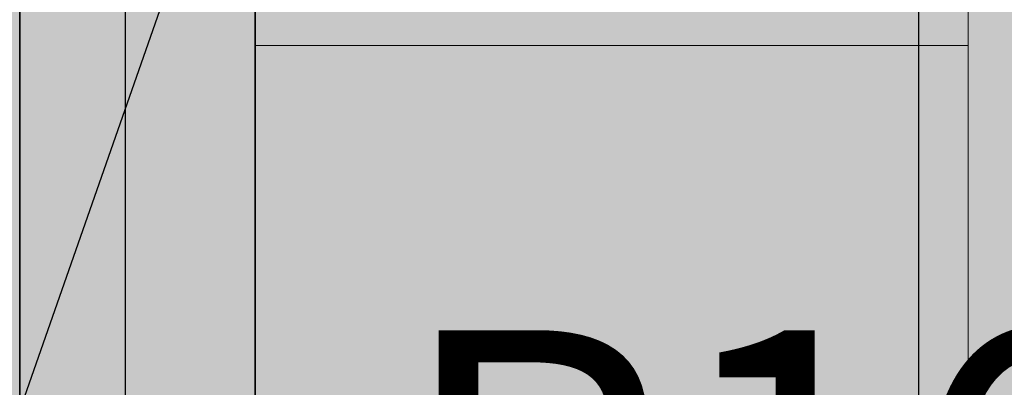
# Model space of a CAD drawing. Units: millimetres. Extents: x 130 to 1021, y 147 to 699.
# Tile 33 of 40: x 487 to 550, y 515 to 539. Entities that reach past the tile are written whole.
import ezdxf

# ---------------------------------------------------------------- set-up
doc = ezdxf.new("R2010")
doc.units = ezdxf.units.MM
doc.header["$MEASUREMENT"] = 0
for name, color, linetype, lineweight in [('A-ANNO-DIMS', 2, 'Continuous', 18), ('A-ELEV', 7, 'Continuous', 35), ('A-ELEV-PATT', 9, 'Continuous', 13), ('A-GLAZ', 4, 'Continuous', 18)]:
    doc.layers.add(name, color=color, linetype=linetype, lineweight=lineweight)
doc.styles.get("Standard").update_dxf_attribs({"font": 'arial.ttf'})
doc.dimstyles.get("Standard").update_dxf_attribs({"dimtxt": 20, "dimasz": 10, "dimexe": 10, "dimexo": 10, "dimgap": 5, "dimtad": 0, "dimtih": 1, "dimtoh": 1, "dimdec": 0, "dimzin": 0, "dimdsep": 46, "dimtxsty": 'Standard', "dimcen": 5, "dimadec": 0, "dimazin": 0, "dimtfac": 1, "dimtdec": 0, "dimtofl": 0, "dimtmove": 0, "dimatfit": 3, "dimfxl": 1, "dimtolj": 1, "dimtzin": 0, "dimarcsym": 0})

# ---------------------------------------------------------------- blocks, each defined once
blk = doc.blocks.new('*D11')
at = {"layer": 'A-ANNO-DIMS', "color": 0, "lineweight": -2, "transparency": 16777216}
for p, q in [((737.374, 648.699), (737.374, 149.739)), ((299.374, 566.947), (299.374, 149.739)), ((309.374, 159.739), (490.857, 159.739)), ((727.374, 159.739), (545.891, 159.739))]:
    blk.add_line(p, q, dxfattribs=at)
at = {"layer": 'A-ANNO-DIMS', "color": 0, "transparency": 16777216}
for points in [[(309.374, 161.406), (309.374, 158.073), (299.374, 159.739)], [(727.374, 161.406), (727.374, 158.073), (737.374, 159.739)]]:
    blk.add_solid(points, dxfattribs=at)
at = {"layer": 'Defpoints', "color": 0, "transparency": 16777216}
for p in [(737.374, 658.699), (299.374, 576.947), (737.374, 159.739)]:
    blk.add_point(p, dxfattribs=at)
at = {"layer": 'A-ANNO-DIMS', "color": 0, "transparency": 16777216, "insert": (518.374, 159.739), "char_height": 20, "attachment_point": 5}
blk.add_mtext('\\A1;438', dxfattribs=at)
blk = doc.blocks.new('*D12')
at = {"layer": 'A-ANNO-DIMS', "color": 0, "lineweight": -2, "transparency": 16777216}
for p, q in [((477.374, 661.947), (265.074, 661.947)), ((275.074, 651.947), (275.074, 438.205)), ((275.074, 194.039), (275.074, 407.782)), ((357.163, 184.039), (265.074, 184.039))]:
    blk.add_line(p, q, dxfattribs=at)
at = {"layer": 'A-ANNO-DIMS', "color": 0, "transparency": 16777216}
for points in [[(273.407, 651.947), (276.74, 651.947), (275.074, 661.947)], [(273.407, 194.039), (276.74, 194.039), (275.074, 184.039)]]:
    blk.add_solid(points, dxfattribs=at)
at = {"layer": 'Defpoints', "color": 0, "transparency": 16777216}
for p in [(275.074, 661.947), (487.374, 661.947), (367.163, 184.039)]:
    blk.add_point(p, dxfattribs=at)
at = {"layer": 'A-ANNO-DIMS', "color": 0, "transparency": 16777216, "insert": (275.074, 422.993), "char_height": 20, "attachment_point": 5}
blk.add_mtext('\\A1;477.9', dxfattribs=at)
blk = doc.blocks.new('*D19')
at = {"layer": 'A-ANNO-DIMS', "color": 0, "lineweight": -2, "transparency": 16777216}
for p, q in [((382.374, 388.947), (382.374, 696.247)), ((414.652, 510.881), (414.652, 696.247)), ((392.374, 686.247), (404.652, 686.247)), ((414.652, 686.247), (424.652, 686.247))]:
    blk.add_line(p, q, dxfattribs=at)
at = {"layer": 'A-ANNO-DIMS', "color": 0, "transparency": 16777216}
for points in [[(392.374, 687.914), (392.374, 684.581), (382.374, 686.247)], [(404.652, 687.914), (404.652, 684.581), (414.652, 686.247)]]:
    blk.add_solid(points, dxfattribs=at)
at = {"layer": 'Defpoints', "color": 0, "transparency": 16777216}
for p in [(414.652, 686.247), (414.652, 500.881), (382.374, 378.947)]:
    blk.add_point(p, dxfattribs=at)
at = {"layer": 'A-ANNO-DIMS', "color": 0, "transparency": 16777216, "insert": (463.411, 686.247), "char_height": 20, "attachment_point": 5}
blk.add_mtext('\\A1;32.28', dxfattribs=at)
blk = doc.blocks.new('*D20')
at = {"layer": 'A-ANNO-DIMS', "color": 0, "lineweight": -2, "transparency": 16777216}
for p, q in [((414.652, 510.881), (414.652, 696.247)), ((432.374, 388.947), (432.374, 696.247)), ((404.652, 686.247), (394.652, 686.247)), ((442.374, 686.247), (452.374, 686.247))]:
    blk.add_line(p, q, dxfattribs=at)
at = {"layer": 'A-ANNO-DIMS', "color": 0, "transparency": 16777216}
for points in [[(404.652, 687.914), (404.652, 684.581), (414.652, 686.247)], [(442.374, 687.914), (442.374, 684.581), (432.374, 686.247)]]:
    blk.add_solid(points, dxfattribs=at)
at = {"layer": 'Defpoints', "color": 0, "transparency": 16777216}
for p in [(432.374, 686.247), (414.652, 500.881), (432.374, 378.947)]:
    blk.add_point(p, dxfattribs=at)
at = {"layer": 'A-ANNO-DIMS', "color": 0, "transparency": 16777216, "insert": (490.075, 686.247), "char_height": 20, "attachment_point": 5}
blk.add_mtext('\\A1;17.72', dxfattribs=at)
blk = doc.blocks.new('*D21')
at = {"layer": 'A-ANNO-DIMS', "color": 0, "lineweight": -2, "transparency": 16777216}
for p, q in [((432.374, 388.947), (432.374, 696.247)), ((447.374, 656.947), (447.374, 696.247)), ((422.374, 686.247), (412.374, 686.247)), ((457.374, 686.247), (467.374, 686.247))]:
    blk.add_line(p, q, dxfattribs=at)
at = {"layer": 'A-ANNO-DIMS', "color": 0, "transparency": 16777216}
for points in [[(422.374, 687.914), (422.374, 684.581), (432.374, 686.247)], [(457.374, 687.914), (457.374, 684.581), (447.374, 686.247)]]:
    blk.add_solid(points, dxfattribs=at)
at = {"layer": 'Defpoints', "color": 0, "transparency": 16777216}
for p in [(447.374, 686.247), (447.374, 646.947), (432.374, 378.947)]:
    blk.add_point(p, dxfattribs=at)
at = {"layer": 'A-ANNO-DIMS', "color": 0, "transparency": 16777216, "insert": (485.832, 686.247), "char_height": 20, "attachment_point": 5}
blk.add_mtext('\\A1;15', dxfattribs=at)
blk = doc.blocks.new('*D22')
at = {"layer": 'A-ANNO-DIMS', "color": 0, "lineweight": -2, "transparency": 16777216}
for p, q in [((447.374, 656.947), (447.374, 696.247)), ((466.767, 403.947), (466.767, 696.247)), ((437.374, 686.247), (427.374, 686.247)), ((476.767, 686.247), (486.767, 686.247))]:
    blk.add_line(p, q, dxfattribs=at)
at = {"layer": 'A-ANNO-DIMS', "color": 0, "transparency": 16777216}
for points in [[(437.374, 687.914), (437.374, 684.581), (447.374, 686.247)], [(476.767, 687.914), (476.767, 684.581), (466.767, 686.247)]]:
    blk.add_solid(points, dxfattribs=at)
at = {"layer": 'Defpoints', "color": 0, "transparency": 16777216}
for p in [(466.767, 686.247), (447.374, 646.947), (466.767, 393.947)]:
    blk.add_point(p, dxfattribs=at)
at = {"layer": 'A-ANNO-DIMS', "color": 0, "transparency": 16777216, "insert": (532.34, 686.247), "char_height": 20, "attachment_point": 5}
blk.add_mtext('\\A1;19.393', dxfattribs=at)
blk = doc.blocks.new('*D23')
at = {"layer": 'A-ANNO-DIMS', "color": 0, "lineweight": -2, "transparency": 16777216}
for p, q in [((466.767, 403.947), (466.767, 696.247)), ((475.988, 209.039), (475.988, 696.247)), ((456.767, 686.247), (446.767, 686.247)), ((485.988, 686.247), (495.988, 686.247))]:
    blk.add_line(p, q, dxfattribs=at)
at = {"layer": 'A-ANNO-DIMS', "color": 0, "transparency": 16777216}
for points in [[(456.767, 687.914), (456.767, 684.581), (466.767, 686.247)], [(485.988, 687.914), (485.988, 684.581), (475.988, 686.247)]]:
    blk.add_solid(points, dxfattribs=at)
at = {"layer": 'Defpoints', "color": 0, "transparency": 16777216}
for p in [(475.988, 686.247), (466.767, 393.947), (475.988, 199.039)]:
    blk.add_point(p, dxfattribs=at)
at = {"layer": 'A-ANNO-DIMS', "color": 0, "transparency": 16777216, "insert": (534.631, 686.247), "char_height": 20, "attachment_point": 5}
blk.add_mtext('\\A1;9.222', dxfattribs=at)
blk = doc.blocks.new('*D24')
at = {"layer": 'A-ANNO-DIMS', "color": 0, "lineweight": -2, "transparency": 16777216}
for p, q in [((475.988, 209.039), (475.988, 696.247)), ((487.374, 671.947), (487.374, 696.247)), ((465.988, 686.247), (455.988, 686.247)), ((497.374, 686.247), (507.374, 686.247))]:
    blk.add_line(p, q, dxfattribs=at)
at = {"layer": 'A-ANNO-DIMS', "color": 0, "transparency": 16777216}
for points in [[(465.988, 687.914), (465.988, 684.581), (475.988, 686.247)], [(497.374, 687.914), (497.374, 684.581), (487.374, 686.247)]]:
    blk.add_solid(points, dxfattribs=at)
at = {"layer": 'Defpoints', "color": 0, "transparency": 16777216}
for p in [(487.374, 686.247), (487.374, 661.947), (475.988, 199.039)]:
    blk.add_point(p, dxfattribs=at)
at = {"layer": 'A-ANNO-DIMS', "color": 0, "transparency": 16777216, "insert": (553.022, 686.247), "char_height": 20, "attachment_point": 5}
blk.add_mtext('\\A1;11.385', dxfattribs=at)
blk = doc.blocks.new('*D25')
at = {"layer": 'A-ANNO-DIMS', "color": 0, "lineweight": -2, "transparency": 16777216}
for p, q in [((487.374, 671.947), (487.374, 696.247)), ((494.102, 506.908), (494.102, 696.247)), ((477.374, 686.247), (467.374, 686.247)), ((504.102, 686.247), (514.102, 686.247))]:
    blk.add_line(p, q, dxfattribs=at)
at = {"layer": 'A-ANNO-DIMS', "color": 0, "transparency": 16777216}
for points in [[(477.374, 687.914), (477.374, 684.581), (487.374, 686.247)], [(504.102, 687.914), (504.102, 684.581), (494.102, 686.247)]]:
    blk.add_solid(points, dxfattribs=at)
at = {"layer": 'Defpoints', "color": 0, "transparency": 16777216}
for p in [(494.102, 686.247), (487.374, 661.947), (494.102, 496.908)]:
    blk.add_point(p, dxfattribs=at)
at = {"layer": 'A-ANNO-DIMS', "color": 0, "transparency": 16777216, "insert": (552.922, 686.247), "char_height": 20, "attachment_point": 5}
blk.add_mtext('\\A1;6.728', dxfattribs=at)
blk = doc.blocks.new('*D26')
at = {"layer": 'A-ANNO-DIMS', "color": 0, "lineweight": -2, "transparency": 16777216}
for p, q in [((494.102, 506.908), (494.102, 696.247)), ((502.374, 593.947), (502.374, 696.247)), ((484.102, 686.247), (474.102, 686.247)), ((512.374, 686.247), (522.374, 686.247))]:
    blk.add_line(p, q, dxfattribs=at)
at = {"layer": 'A-ANNO-DIMS', "color": 0, "transparency": 16777216}
for points in [[(484.102, 687.914), (484.102, 684.581), (494.102, 686.247)], [(512.374, 687.914), (512.374, 684.581), (502.374, 686.247)]]:
    blk.add_solid(points, dxfattribs=at)
at = {"layer": 'Defpoints', "color": 0, "transparency": 16777216}
for p in [(502.374, 686.247), (502.374, 583.947), (494.102, 496.908)]:
    blk.add_point(p, dxfattribs=at)
at = {"layer": 'A-ANNO-DIMS', "color": 0, "transparency": 16777216, "insert": (561.03, 686.247), "char_height": 20, "attachment_point": 5}
blk.add_mtext('\\A1;8.272', dxfattribs=at)
blk = doc.blocks.new('*D27')
at = {"layer": 'A-ANNO-DIMS', "color": 0, "lineweight": -2, "transparency": 16777216}
for p, q in [((502.374, 593.947), (502.374, 696.247)), ((544.635, 396.264), (544.635, 696.247)), ((512.374, 686.247), (534.635, 686.247)), ((544.635, 686.247), (554.635, 686.247))]:
    blk.add_line(p, q, dxfattribs=at)
at = {"layer": 'A-ANNO-DIMS', "color": 0, "transparency": 16777216}
for points in [[(512.374, 687.914), (512.374, 684.581), (502.374, 686.247)], [(534.635, 687.914), (534.635, 684.581), (544.635, 686.247)]]:
    blk.add_solid(points, dxfattribs=at)
at = {"layer": 'Defpoints', "color": 0, "transparency": 16777216}
for p in [(544.635, 686.247), (502.374, 583.947), (544.635, 386.264)]:
    blk.add_point(p, dxfattribs=at)
at = {"layer": 'A-ANNO-DIMS', "color": 0, "transparency": 16777216, "insert": (593.776, 686.247), "char_height": 20, "attachment_point": 5}
blk.add_mtext('\\A1;42.26', dxfattribs=at)
blk = doc.blocks.new('*D28')
at = {"layer": 'A-ANNO-DIMS', "color": 0, "lineweight": -2, "transparency": 16777216}
for p, q in [((544.635, 396.264), (544.635, 696.247)), ((552.374, 593.947), (552.374, 696.247)), ((534.635, 686.247), (524.635, 686.247)), ((562.374, 686.247), (572.374, 686.247))]:
    blk.add_line(p, q, dxfattribs=at)
at = {"layer": 'A-ANNO-DIMS', "color": 0, "transparency": 16777216}
for points in [[(534.635, 687.914), (534.635, 684.581), (544.635, 686.247)], [(562.374, 687.914), (562.374, 684.581), (552.374, 686.247)]]:
    blk.add_solid(points, dxfattribs=at)
at = {"layer": 'Defpoints', "color": 0, "transparency": 16777216}
for p in [(552.374, 686.247), (552.374, 583.947), (544.635, 386.264)]:
    blk.add_point(p, dxfattribs=at)
at = {"layer": 'A-ANNO-DIMS', "color": 0, "transparency": 16777216, "insert": (611.057, 686.247), "char_height": 20, "attachment_point": 5}
blk.add_mtext('\\A1;7.738', dxfattribs=at)
blk = doc.blocks.new('*D65')
at = {"layer": 'A-ANNO-DIMS', "color": 0, "lineweight": -2, "transparency": 16777216}
for p, q in [((495.463, 509.127), (472.508, 423.108)), ((505.463, 509.127), (495.463, 509.127)), ((427.374, 248.979), (427.374, 258.979)), ((422.374, 253.979), (432.374, 253.979))]:
    blk.add_line(p, q, dxfattribs=at)
at = {"layer": 'A-ANNO-DIMS', "color": 0, "transparency": 16777216}
blk.add_solid([(470.898, 423.538), (474.118, 422.679), (469.93, 413.447)], dxfattribs=at)
at = {"layer": 'Defpoints', "color": 0, "transparency": 16777216}
for p in [(469.93, 413.447), (427.374, 253.979)]:
    blk.add_point(p, dxfattribs=at)
at = {"layer": 'A-ANNO-DIMS', "color": 0, "transparency": 16777216, "insert": (561.623, 509.127), "char_height": 20, "attachment_point": 5}
blk.add_mtext('\\A1;R165.05', dxfattribs=at)
blk = doc.blocks.new('*D69')
at = {"layer": 'A-ANNO-DIMS', "color": 0, "lineweight": -2, "transparency": 16777216}
for p, q in [((507.746, 572.261), (483.091, 501.813)), ((517.746, 572.261), (507.746, 572.261)), ((433.191, 354.23), (433.191, 364.23)), ((428.191, 359.23), (438.191, 359.23))]:
    blk.add_line(p, q, dxfattribs=at)
at = {"layer": 'A-ANNO-DIMS', "color": 0, "transparency": 16777216}
blk.add_solid([(481.518, 502.363), (484.664, 501.262), (479.788, 492.374)], dxfattribs=at)
at = {"layer": 'Defpoints', "color": 0, "transparency": 16777216}
for p in [(479.788, 492.374), (433.191, 359.23)]:
    blk.add_point(p, dxfattribs=at)
at = {"layer": 'A-ANNO-DIMS', "color": 0, "transparency": 16777216, "insert": (573.824, 572.261), "char_height": 20, "attachment_point": 5}
blk.add_mtext('\\A1;R141.06', dxfattribs=at)
blk = doc.blocks.new('*D71')
at = {"layer": 'A-ANNO-DIMS', "color": 0, "lineweight": -2, "transparency": 16777216}
for p, q in [((492.108, 581.609), (472.542, 512.666)), ((502.108, 581.609), (492.108, 581.609)), ((432.65, 367.109), (432.65, 377.109)), ((427.65, 372.109), (437.65, 372.109))]:
    blk.add_line(p, q, dxfattribs=at)
at = {"layer": 'A-ANNO-DIMS', "color": 0, "transparency": 16777216}
blk.add_solid([(470.938, 513.121), (474.145, 512.211), (469.812, 503.046)], dxfattribs=at)
at = {"layer": 'Defpoints', "color": 0, "transparency": 16777216}
for p in [(469.812, 503.046), (432.65, 372.109)]:
    blk.add_point(p, dxfattribs=at)
at = {"layer": 'A-ANNO-DIMS', "color": 0, "transparency": 16777216, "insert": (548.493, 581.609), "char_height": 20, "attachment_point": 5}
blk.add_mtext('\\A1;R136.1', dxfattribs=at)
blk = doc.blocks.new('*D72')
at = {"layer": 'A-ANNO-DIMS', "color": 0, "lineweight": -2, "transparency": 16777216}
for p, q in [((460.658, 573.64), (451.279, 503.49)), ((470.658, 573.64), (460.658, 573.64)), ((432.115, 355.142), (432.115, 365.142)), ((427.115, 360.142), (437.115, 360.142))]:
    blk.add_line(p, q, dxfattribs=at)
at = {"layer": 'A-ANNO-DIMS', "color": 0, "transparency": 16777216}
blk.add_solid([(449.628, 503.711), (452.931, 503.27), (449.954, 493.579)], dxfattribs=at)
at = {"layer": 'Defpoints', "color": 0, "transparency": 16777216}
for p in [(449.954, 493.579), (432.115, 360.142)]:
    blk.add_point(p, dxfattribs=at)
at = {"layer": 'A-ANNO-DIMS', "color": 0, "transparency": 16777216, "insert": (526.64, 573.64), "char_height": 20, "attachment_point": 5}
blk.add_mtext('\\A1;R134.62', dxfattribs=at)

msp = doc.modelspace()

# ---------------------------------------------------------------- hatches: boundary and pattern name
at = {"layer": 'A-ELEV-PATT'}
h = msp.add_hatch(color=256, dxfattribs=at)
h.paths.add_polyline_path([(327.3738, 569.884), (327.3738, 573.9473), (307.3738, 573.9473), (307.3738, 476.9473), (327.3738, 476.9473), (327.3738, 480.95)])
h.paths.add_polyline_path([(486.7667, 386.2639), (486.7667, 393.9473), (466.7667, 393.9473), (466.7667, 357.2114), (466.7667, 311.9335, 0.0342703), (486.7667, 308.4637)])
h.paths.add_polyline_path([(486.7667, 308.4637, -0.0342703), (466.7667, 311.9335), (466.7667, 273.9473), (486.7667, 273.9473)])
h.paths.add_polyline_path([(389.3738, 351.5473), (396.7693, 351.5473, -0.007027), (393.8774, 354.5473), (389.3738, 354.5473), (389.3738, 359.5775, -0.0190302), (382.3738, 368.424), (382.3738, 249.5473), (432.3738, 249.5473), (432.3738, 325.067, -0.0057673), (429.3738, 326.709), (429.3738, 257.5473), (426.3738, 257.5473), (426.3738, 328.4428, -0.0059254), (423.3738, 330.272), (423.3738, 315.7473), (389.3738, 315.7473), (389.3738, 332.1473), (420.4552, 332.1473, -0.008951), (416.0768, 335.1473), (389.3738, 335.1473)])
h.paths.add_polyline_path([(389.3738, 312.7473), (423.3738, 312.7473), (423.3738, 296.3473), (389.3738, 296.3473)], flags=16)
h.paths.add_polyline_path([(389.3738, 293.3473), (423.3738, 293.3473), (423.3738, 276.9473), (389.3738, 276.9473)], flags=16)
h.paths.add_polyline_path([(389.3738, 273.9473), (423.3738, 273.9473), (423.3738, 257.5473), (389.3738, 257.5473)], flags=16)
h.paths.add_polyline_path([(432.3738, 378.9473), (382.3738, 378.9473), (382.3738, 368.424, 0.0190302), (389.3738, 359.5775), (389.3738, 370.9473), (423.3738, 370.9473), (423.3738, 354.5473), (393.8774, 354.5473, 0.007027), (396.7693, 351.5473), (423.3738, 351.5473), (423.3738, 335.1473), (416.0768, 335.1473, 0.008951), (420.4552, 332.1473), (423.3738, 332.1473), (423.3738, 330.272, 0.0059254), (426.3738, 328.4428), (426.3738, 370.9473), (429.3738, 370.9473), (429.3738, 326.709, 0.0057673), (432.3738, 325.067)])
h.paths.add_polyline_path([(466.7667, 357.2114), (466.7667, 393.9473), (447.3738, 393.9473), (447.3738, 357.2114), (447.3738, 318.1243, 0.0063261), (450.8779, 316.785), (450.8779, 331.5915), (463.5608, 331.5915), (463.5608, 312.7571, 0.005582), (466.7667, 311.9335)])
h.paths.add_polyline_path([(450.8779, 334.5915), (450.8779, 360.0915), (463.5608, 360.0915), (463.5608, 334.5915)], flags=16)
h.paths.add_polyline_path([(450.8779, 363.0915), (450.8779, 388.6449), (463.5608, 388.6449), (463.5608, 363.0915)], flags=16)
h.paths.add_polyline_path([(466.7667, 311.9335, -0.005582), (463.5608, 312.7571), (463.5608, 306.0915), (450.8779, 306.0915), (450.8779, 316.785, -0.0063261), (447.3738, 318.1243), (447.3738, 273.9473), (466.7667, 273.9473)])
h.paths.add_polyline_path([(450.8779, 303.0915), (463.5608, 303.0915), (463.5608, 277.5915), (450.8779, 277.5915)], flags=16)
h.paths.add_polyline_path([(552.3738, 357.2114), (552.3738, 393.9473), (486.7667, 393.9473), (486.7667, 386.2639), (544.6354, 386.2639), (544.6354, 280.6619), (486.7667, 280.6619), (486.7667, 273.9473), (552.3738, 273.9473)])
h.paths.add_polyline_path([(487.3738, 583.9473), (472.3738, 580.1973), (472.3738, 507.0765), (472.3738, 505.4251, -0.0056452), (475.3738, 504.4942), (475.3738, 506.3543), (475.3738, 511.9473), (484.3738, 511.9473), (484.3738, 503.8134), (484.3738, 501.2439, -0.0058357), (487.3738, 500.0015)])
h.paths.add_polyline_path([(484.3738, 578.0434), (484.3738, 548.9473), (475.3738, 548.9473), (475.3738, 575.7934)], flags=16)
h.paths.add_polyline_path([(484.3738, 546.9473), (484.3738, 513.9473), (475.3738, 513.9473), (475.3738, 518.7148), (475.3738, 546.9473)], flags=16)
for points in [[(502.3738, 583.9473), (487.3738, 583.9473), (487.3738, 500.0015, -0.0133113), (494.1023, 496.908), (494.1023, 476.9473), (502.3738, 476.9473)], [(502.3738, 583.9473), (502.3738, 577.3739), (547.7773, 577.3739), (547.7773, 481.7432), (502.3738, 481.7432), (502.3738, 476.9473), (552.3738, 476.9473), (552.3738, 583.9473)]]:
    msp.add_hatch(color=256, dxfattribs=at).paths.add_polyline_path(points)
h = msp.add_hatch(color=256, dxfattribs=at)
h.dxf.hatch_style = 1
h.paths.add_polyline_path([(502.3738, 566.2111), (502.3738, 548.9473), (547.7773, 548.9473), (547.7773, 566.2111)])
h.paths.add_polyline_path([(502.3738, 546.9473), (502.3738, 537.2685), (547.7773, 537.2685), (547.7773, 546.9473)])
h.paths.add_polyline_path([(486.7667, 360.9454), (486.7667, 336.9454), (544.6354, 336.9453), (544.6354, 360.9453)])
h.paths.add_polyline_path([(496.0546, 377.43), (486.7667, 370.4028), (486.7667, 363.9454), (544.6354, 363.9453), (544.6354, 377.43)])
h = msp.add_hatch(color=256, dxfattribs=at)
h.dxf.hatch_style = 1
h.paths.add_polyline_path([(364.0891, 218.0087), (361.0152, 221.978), (361.0152, 236.978), (357.9413, 240.9473), (357.9413, 195.9473), (367.163, 184.0395), (367.163, 199.0395), (364.0891, 203.0087)])
h.paths.add_polyline_path([(502.3738, 537.2685), (502.3738, 513.9473), (547.7773, 513.9473), (547.7773, 537.2685)])
h.paths.add_polyline_path([(502.3738, 511.9473), (502.3738, 481.7432), (547.7773, 481.7432), (547.7773, 511.9473)])
h.paths.add_polyline_path([(327.3738, 529.7), (327.3738, 509.9473), (363.922, 509.9473), (363.922, 529.7)])
h.paths.add_polyline_path([(327.3738, 507.9473), (327.3738, 480.95), (363.922, 480.95), (363.922, 507.9473)])

# ---------------------------------------------------------------- linework, layer by layer
at = {"layer": 'A-ELEV'}
for p, q in [((487.3738, 500.0015), (487.3738, 646.9473)), ((502.3738, 583.9473), (502.3738, 476.9473))]:
    msp.add_line(p, q, dxfattribs=at)
at = {"layer": 'A-GLAZ'}
msp.add_line((502.3738, 537.2685), (547.7773, 537.2685), dxfattribs=at)
msp.add_lwpolyline([(502.3738, 481.7432), (547.7773, 481.7432), (547.7773, 577.3739), (502.3738, 577.3739)], dxfattribs=at)

# ---------------------------------------------------------------- dimensions: what is measured, and where the dimension line sits
at = {"layer": 'A-ANNO-DIMS'}
for base, p1, p2, override, picture, middle in [((414.6525, 686.2473), (382.3738, 378.9473), (414.6525, 500.8811), {"dimdec": 2, "dimlfac": 1, "dimrnd": 0, "dimzin": 0, "dimdsep": 46, "dimlunit": 2}, '*D19', (463.411, 686.2473)), ((432.3738, 686.2473), (414.6525, 500.8811), (432.3738, 378.9473), {"dimdec": 2, "dimlfac": 1, "dimrnd": 0, "dimzin": 0, "dimdsep": 46, "dimlunit": 2}, '*D20', (490.075, 686.2473)), ((447.3738, 686.2473), (432.3738, 378.9473), (447.3738, 646.9473), {"dimdec": 0, "dimlfac": 1, "dimrnd": 0, "dimzin": 0, "dimdsep": 46, "dimlunit": 2}, '*D21', (485.8322, 686.2473)), ((466.7667, 686.2473), (447.3738, 646.9473), (466.7667, 393.9473), {"dimdec": 3, "dimlfac": 1, "dimrnd": 0, "dimzin": 0, "dimdsep": 46, "dimlunit": 2}, '*D22', (532.3397, 686.2473)), ((475.9885, 686.2473), (466.7667, 393.9473), (475.9885, 199.0395), {"dimdec": 3, "dimlfac": 1, "dimrnd": 0, "dimzin": 0, "dimdsep": 46, "dimlunit": 2}, '*D23', (534.631, 686.2473)), ((487.3738, 686.2473), (475.9885, 199.0395), (487.3738, 661.9473), {"dimdec": 3, "dimlfac": 1, "dimrnd": 0, "dimzin": 0, "dimdsep": 46, "dimlunit": 2}, '*D24', (553.0218, 686.2473)), ((494.10227, 686.2473), (487.37378, 661.9473), (494.10227, 496.90803), {"dimdec": 3, "dimlfac": 1, "dimrnd": 0, "dimzin": 0, "dimdsep": 46, "dimlunit": 2}, '*D25', (552.92219, 686.2473)), ((502.37378, 686.2473), (494.10227, 496.90803), (502.37378, 583.9473), {"dimdec": 3, "dimlfac": 1, "dimrnd": 0, "dimzin": 0, "dimdsep": 46, "dimlunit": 2}, '*D26', (561.02999, 686.2473)), ((544.6354, 686.2473), (502.3738, 583.9473), (544.6354, 386.2639), {"dimdec": 2, "dimlfac": 1, "dimrnd": 0, "dimzin": 0, "dimdsep": 46, "dimlunit": 2}, '*D27', (593.776, 686.2473)), ((552.3738, 686.2473), (544.6354, 386.2639), (552.3738, 583.9473), {"dimdec": 3, "dimlfac": 1, "dimrnd": 0, "dimzin": 0, "dimdsep": 46, "dimlunit": 2}, '*D28', (611.0573, 686.2473)), ((737.3738, 159.7395), (299.3738, 576.9473), (737.3738, 658.6988), {"dimdec": 0, "dimlfac": 1, "dimrnd": 0, "dimzin": 0, "dimdsep": 46, "dimlunit": 2}, '*D11', (518.3738, 159.7395))]:
    dim = msp.add_linear_dim(base=base, p1=p1, p2=p2, dimstyle='Standard', override=override, dxfattribs=at)
    dim.commit()
    dim.dimension.update_dxf_attribs({"geometry": picture, "text_midpoint": middle})
dim = msp.add_linear_dim(base=(275.0738, 661.9473), p1=(367.163, 184.0395), p2=(487.3738, 661.9473), angle=90, dimstyle='Standard', override={"dimdec": 1, "dimlfac": 1, "dimrnd": 0, "dimzin": 0, "dimdsep": 46, "dimlunit": 2}, dxfattribs=at)
dim.commit()
dim.dimension.update_dxf_attribs({"geometry": '*D12', "text_midpoint": (275.0738, 422.9934)})
for center, mpoint, override, picture, middle in [((432.6505, 372.1087), (469.8116, 503.0461), {"dimdec": 1, "dimlfac": 1, "dimrnd": 0, "dimzin": 0, "dimdsep": 46, "dimlunit": 2}, '*D71', (548.493, 581.6085)), ((432.115, 360.1423), (449.9544, 493.5786), {"dimdec": 2, "dimlfac": 1, "dimrnd": 0, "dimzin": 0, "dimdsep": 46, "dimlunit": 2}, '*D72', (526.6403, 573.6404)), ((433.1906, 359.2304), (479.788, 492.3743), {"dimdec": 2, "dimlfac": 1, "dimrnd": 0, "dimzin": 0, "dimdsep": 46, "dimlunit": 2}, '*D69', (573.8242, 572.2606)), ((427.3738, 253.9788), (469.9297, 413.4465), {"dimdec": 2, "dimlfac": 1, "dimrnd": 0, "dimzin": 0, "dimdsep": 46, "dimlunit": 2}, '*D65', (561.6228, 509.1272))]:
    dim = msp.add_radius_dim(center=center, mpoint=mpoint, dimstyle='Standard', override=override, dxfattribs=at)
    dim.commit()
    dim.dimension.update_dxf_attribs({"geometry": picture, "text_midpoint": middle, "dimtype": 164})

doc.saveas('drawing.dxf')
